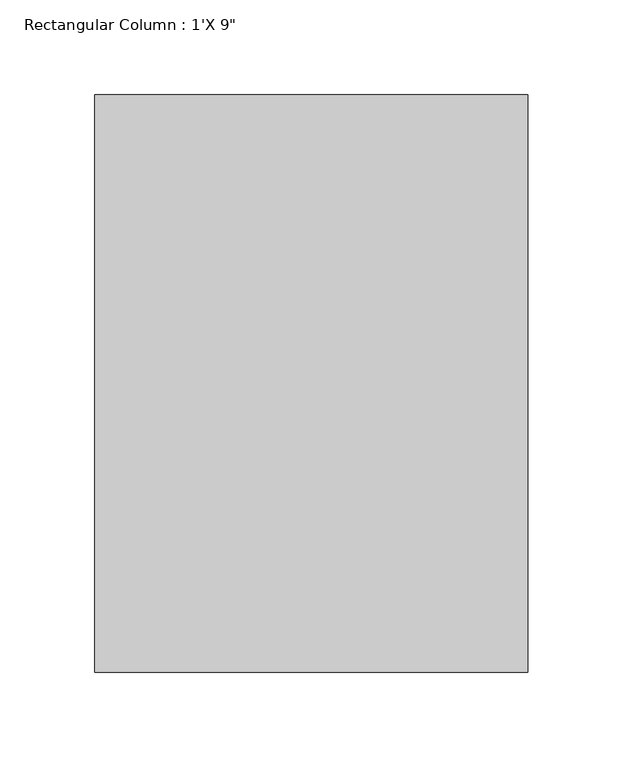
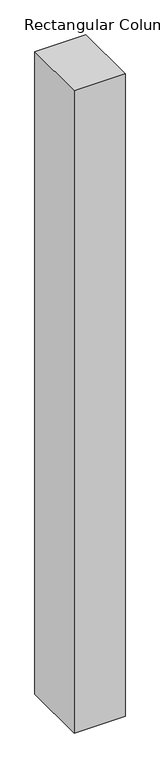
"""IFC4 building model written with IfcOpenShell, lengths in millimetres: column geometry."""

from ifc_helpers import new_model, si_unit, frame, origin, place, context, project, spatial, polyline, outline, extrude, source, transform, mapped, element, save


def column_efe9d5a4(model_context):
    return source(origin(), model_context, "Body", "SweptSolid", [
        extrude(outline(polyline([(114.3, 152.4), (114.3, -152.4), (-114.3, -152.4), (-114.3, 152.4), (114.3, 152.4)])), frame((0.0, 0.0, 16002.0), z_axis=(0.0, 0.0, 1.0), x_axis=(1.0, 0.0, 0.0)), (0.0, 0.0, 1.0), 3048.0),
    ])


if __name__ == "__main__":
    model = new_model("IFC4")
    model_context = context("Model", 3, world=origin())
    ifc_project = project(units=[si_unit("LENGTHUNIT", "METRE", prefix="MILLI")], contexts=[model_context])
    site = spatial("IfcSite", under=ifc_project)
    building = spatial("IfcBuilding", under=site)
    placement = place(None, origin())
    column_shape = column_efe9d5a4(model_context)
    element("IfcColumn", 1, ObjectType="Rectangular Column : 1'X 9\"", at=placement, inside=building, context=model_context, shape_type="MappedRepresentation", body=[
        mapped(column_shape, transform((0.0, 0.0, 0.0), x_axis=(1.0, 0.0, 0.0), y_axis=(0.0, 1.0, 0.0), z_axis=(0.0, 0.0, 1.0))),
    ])
    save(model, "model.ifc")

# Revit data of these elements
# Type "Rectangular Column : 1'X 9\""
#   Assembly Code = "B1010200"
#   Depth = 1' - 0"
#   Offset Base = 0' - 0"
#   Offset Top = 0' - 0"
#   Width = 0' - 9"
#   Material = none
